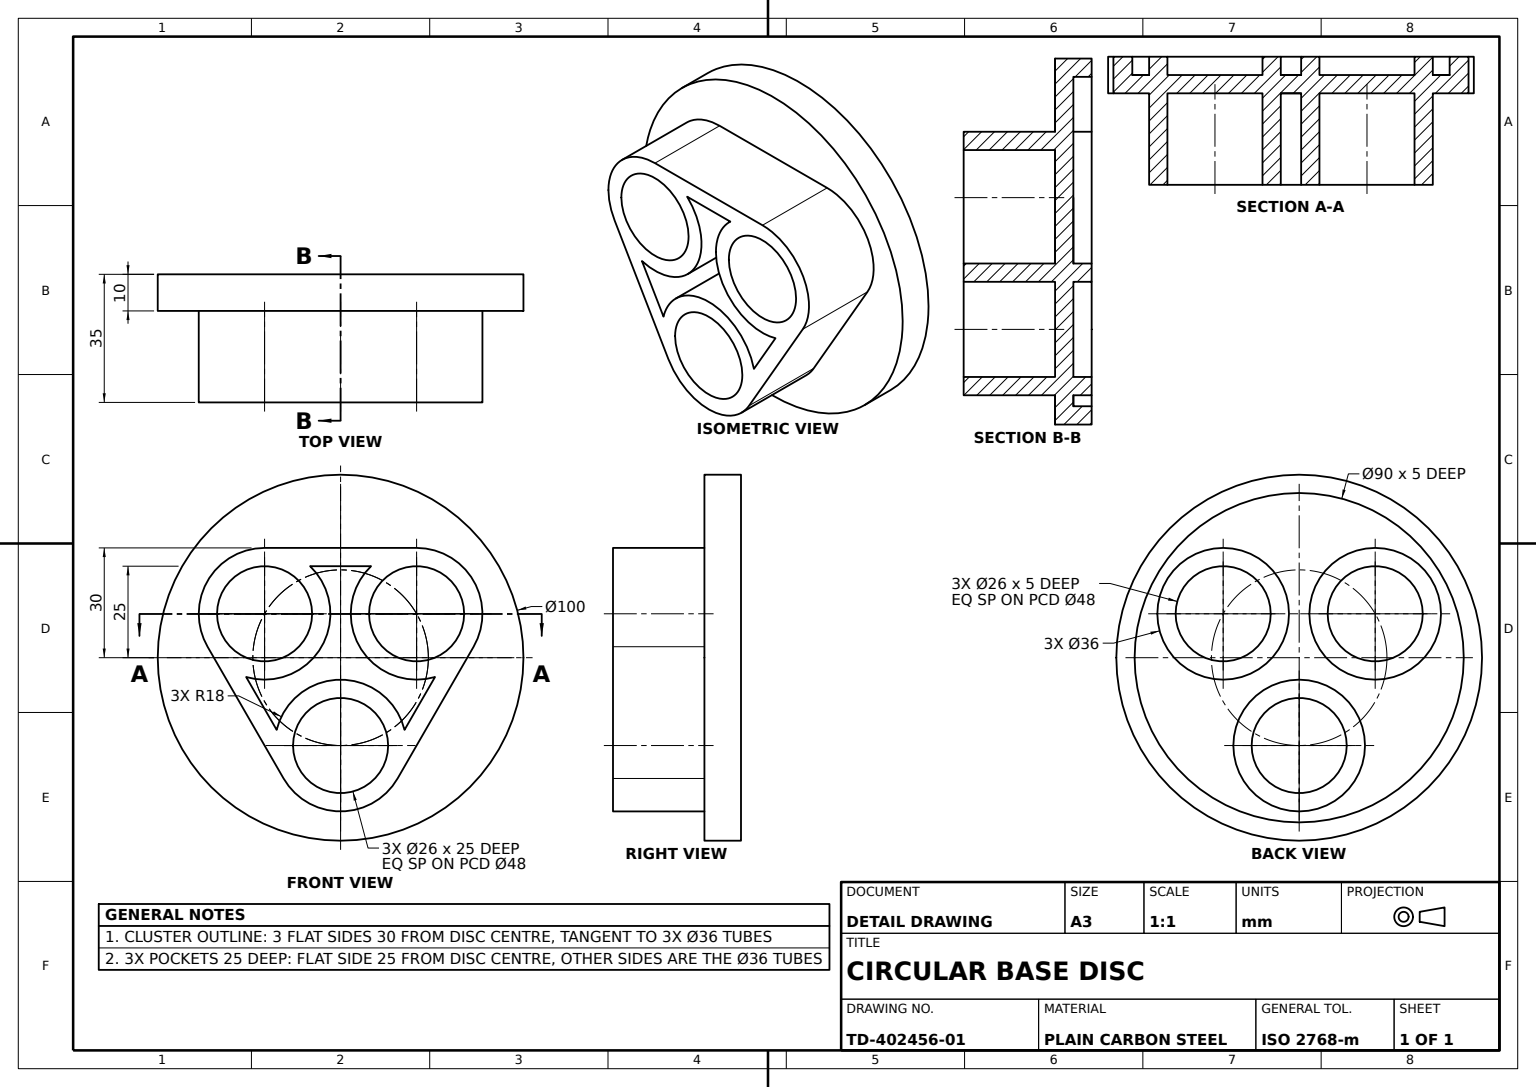
SolidWorks part; units mm, degrees
material "Plain Carbon Steel"
ref_plane "Front Plane" through (0, 0, 0) normal (0, 0, 1) x (1, 0, 0)
ref_plane "Top Plane" through (0, 0, 0) normal (0, 1, 0) x (1, 0, 0)
ref_plane "Right Plane" through (0, 0, 0) normal (1, 0, 0) x (0, 0, -1)
sketch "Flange Profile Ø100" plane through (0, 0, 0) normal (0, 0, 1) x (1, 0, 0)
  circle A0 centre (0, 0) radius 50
  dimension "D1" = 100
extrude "Flange Ø100x10" add sketch "Flange Profile Ø100" along normal blind 10
sketch "Tube Cluster Boss Profile" plane through (0, 0, 10) normal (0, 0, 1) x (1, 0, 0)
  line L0 (0, 50) -> (0, -50)
  line L1 (0, 0) -> (20.7846, 12)
  line L2 (0, 0) -> (24, 0)
  line L3 (0, 0) -> (-24, 0)
  line L4 (0, 0) -> (-20.7846, 12)
  line L5 (-20.7846, 30) -> (20.7846, 30)
  line L6 (-36.3731, 3) -> (-15.5885, -33)
  line L7 (36.3731, 3) -> (15.5885, -33)
  line L8 (0, 30) -> (0, 25)
  line L9 (-21.6506, -12.5) -> (-25.818, -5.2819)
  line L10 (-21.6506, -12.5) -> (-17.4833, -19.7181)
  line L11 (21.6506, -12.5) -> (25.818, -5.2819)
  line L12 (21.6506, -12.5) -> (17.4833, -19.7181)
  line L13 (0, 25) -> (8.3347, 25)
  line L14 (0, 25) -> (-8.3347, 25)
  line L15 (21.6506, -12.5) -> (25.9808, -15)
  line L16 (-25.9808, -15) -> (-21.6506, -12.5)
  circle A0 centre (0, 0) radius 50 construction
  circle A1 centre (0, 0) radius 24 construction
  circle A2 centre (-20.7846, 12) radius 18
  circle A3 centre (0, -24) radius 18
  circle A4 centre (20.7846, 12) radius 18
  circle A5 centre (-20.7846, 12) radius 13
  circle A6 centre (20.7846, 12) radius 13
  circle A7 centre (0, -24) radius 13
  dimension "D1" = 48
  dimension "D4" = 36
  dimension "D5" = 36
  dimension "D6" = 36
  dimension "D7" = 26
  dimension "D8" = 26
  dimension "D9" = 26
  dimension "D2" = 30
  dimension "D3" = 18
  dimension "D10" = 5
  dimension "D11" = 7.2181
  dimension "D12" = 8.3347
  dimension "D13" = 21.6506
  dimension "D14" = 13
extrude "Tube Cluster Boss" add sketch "Tube Cluster Boss Profile" along normal blind 25 contours A5 L4 A2 L3 | A5 L3 A2 L4 | A2 L6 L16 L9 | A3 L10 L16 L6 | A7 L0 A3 | A7 L0 A3 | A3 L7 L15 L12 | A4 L11 L15 L7 | A6 L2 A4 L1 | A6 L1 A4 L2 | A4 L5 L0 L13 | A2 L14 L0 L5
sketch "Flange Recess Profile Ø90" plane through (0, 0, 0) normal (0, 0, -1) x (-1, 0, 0)
  circle A0 centre (0, 0) radius 45
  dimension "D1" = 90
extrude "Flange Recess Ø90x5" cut sketch "Flange Recess Profile Ø90" against normal blind 5
sketch "Tube Profiles 3xØ36-Ø26" plane through (0, 0, 35) normal (0, 0, 1) x (1, 0, 0)
  circle A0 centre (20.7846, 12) radius 18
  circle A1 centre (20.7846, 12) radius 13
  circle A2 centre (-20.7846, 12) radius 18
  circle A3 centre (-20.7846, 12) radius 13
  circle A4 centre (0, -24) radius 13
  circle A5 centre (0, -24) radius 18
  dimension "D1" = 36
  dimension "D2" = 36
  dimension "D3" = 36
  dimension "D4" = 26
  dimension "D5" = 26
  dimension "D6" = 26
extrude "Hollow Tubes 3xØ36" add sketch "Tube Profiles 3xØ36-Ø26" against normal blind 35
